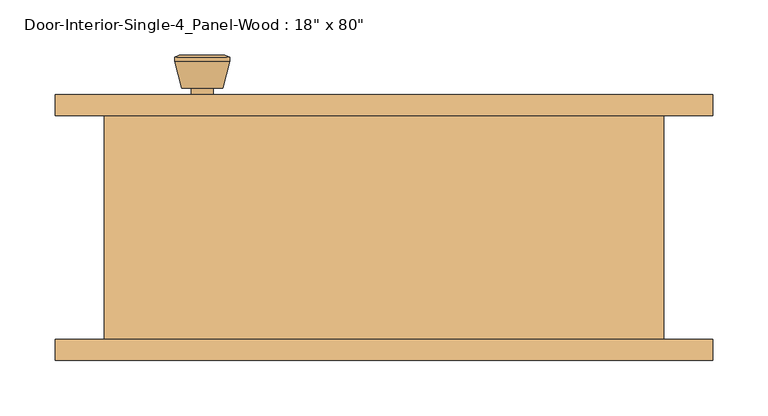
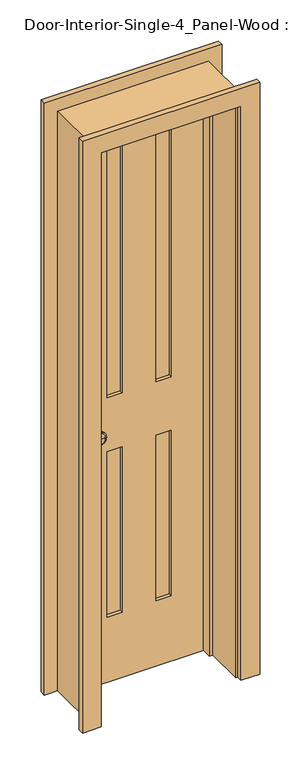
"""IFC4 building model written with IfcOpenShell, lengths in millimetres: door geometry."""

from ifc_helpers import new_model, si_unit, point, frame, frame_2d, origin, place, context, project, spatial, polyline, circle_curve, trimmed, segment, composite_curve, outline, extrude, faceted_brep, source, transform, mapped, element, save
from ifc_brep_helpers import plane_surface, cylinder_surface, revolved_surface, advanced_brep


def door_14995b39(model_context):
    return source(origin(), model_context, "Body", "SolidModel", [
        advanced_brep(
        [(-165.1, 57.5, 914.4), (-155.1, 57.5, 914.4), (-175.1, 57.5, 914.4), (-144.6241324, 8.5, 914.4), (-165.1, 8.5, 914.4), (-185.5758676, 8.5, 914.4), (-140.1, 10.3278681, 914.4), (-190.1, 10.3278681, 914.4), (-140.1, 13.7915463, 914.4), (-190.1, 13.7915463, 914.4), (-146.463764, 38.5, 914.4), (-183.736236, 38.5, 914.4), (-155.1, 38.5, 914.4), (-175.1, 38.5, 914.4)],
        [
            (0, 1),
            (1, 2, circle_curve(frame((-165.1, 57.5, 914.4), z_axis=(0.0, 1.0, 0.0), x_axis=(-1.0, 0.0, 0.0)), 10.0)),
            (2, 0),
            (2, 1, circle_curve(frame((-165.1, 57.5, 914.4), z_axis=(0.0, 1.0, 0.0), x_axis=(-1.0, 0.0, 0.0)), 10.0)),
            (3, 4),
            (4, 5),
            (5, 3, circle_curve(frame((-165.1, 8.5, 914.4), z_axis=(0.0, -1.0, 0.0), x_axis=(-1.0, 0.0, 0.0)), 20.4758676)),
            (3, 5, circle_curve(frame((-165.1, 8.5, 914.4), z_axis=(0.0, -1.0, 0.0), x_axis=(-1.0, 0.0, 0.0)), 20.4758676)),
            (6, 3),
            (5, 7),
            (7, 6, circle_curve(frame((-165.1, 10.3278681, 914.4), z_axis=(0.0, -1.0, 0.0), x_axis=(-1.0, 0.0, 0.0)), 25.0)),
            (6, 7, circle_curve(frame((-165.1, 10.3278681, 914.4), z_axis=(0.0, -1.0, 0.0), x_axis=(-1.0, 0.0, 0.0)), 25.0)),
            (8, 6),
            (7, 9),
            (9, 8, circle_curve(frame((-165.1, 13.7915463, 914.4), z_axis=(0.0, -1.0, 0.0), x_axis=(-1.0, 0.0, 0.0)), 25.0)),
            (8, 9, circle_curve(frame((-165.1, 13.7915463, 914.4), z_axis=(0.0, -1.0, 0.0), x_axis=(-1.0, 0.0, 0.0)), 25.0)),
            (10, 8),
            (9, 11),
            (11, 10, circle_curve(frame((-165.1, 38.5, 914.4), z_axis=(0.0, -1.0, 0.0), x_axis=(-1.0, 0.0, 0.0)), 18.636236)),
            (10, 11, circle_curve(frame((-165.1, 38.5, 914.4), z_axis=(0.0, -1.0, 0.0), x_axis=(-1.0, 0.0, 0.0)), 18.636236)),
            (12, 10),
            (11, 13),
            (13, 12, circle_curve(frame((-165.1, 38.5, 914.4), z_axis=(0.0, -1.0, 0.0), x_axis=(-1.0, 0.0, 0.0)), 10.0)),
            (12, 13, circle_curve(frame((-165.1, 38.5, 914.4), z_axis=(0.0, -1.0, 0.0), x_axis=(-1.0, 0.0, 0.0)), 10.0)),
            (1, 12),
            (13, 2),
        ],
        [
            plane_surface(frame((-165.1, 57.5, 914.4), z_axis=(0.0, 1.0, 0.0), x_axis=(-1.0, 0.0, 0.0))),
            plane_surface(frame((-165.1, 8.5, 914.4), z_axis=(0.0, -1.0, 0.0), x_axis=(-1.0, 0.0, 0.0))),
            revolved_surface(polyline([(-185.5758676, 8.5, 914.4), (-190.1, 10.3278681, 914.4)]), (-165.1, 57.5, 914.4), (0.0, 1.0, 0.0)),
            cylinder_surface(frame((-165.1, 57.5, 914.4), z_axis=(0.0, 1.0, 0.0), x_axis=(-1.0, 0.0, 0.0)), 25.0),
            revolved_surface(polyline([(-190.1, 13.7915463, 914.4), (-183.736236, 38.5, 914.4)]), (-165.1, 57.5, 914.4), (0.0, 1.0, 0.0)),
            plane_surface(frame((-165.1, 38.5, 914.4), z_axis=(0.0, 1.0, 0.0), x_axis=(-1.0, 0.0, 0.0))),
            cylinder_surface(frame((-165.1, 57.5, 914.4), z_axis=(0.0, 1.0, 0.0), x_axis=(-1.0, 0.0, 0.0)), 10.0),
        ],
        [
            (0, [[1, 2, 3]]),
            (0, [[-3, 4, -1]]),
            (1, [[5, 6, 7]]),
            (1, [[-6, -5, 8]]),
            (2, [[9, -7, 10, 11]]),
            (2, [[-10, -8, -9, 12]]),
            (3, [[13, -11, 14, 15]]),
            (3, [[-14, -12, -13, 16]]),
            (4, [[17, -15, 18, 19]]),
            (4, [[-18, -16, -17, 20]]),
            (5, [[21, -19, 22, 23]]),
            (5, [[-22, -20, -21, 24]]),
            (6, [[25, -23, 26, -2]]),
            (6, [[-26, -24, -25, -4]]),
        ],
    ),
        extrude(outline(composite_curve([segment(trimmed(circle_curve(frame_2d((914.4, -165.1)), 30.0), [point((914.4, -195.1))], [point((914.4, -135.1))], False, "CARTESIAN"), True, "CONTINUOUS"), segment(trimmed(circle_curve(frame_2d((914.4, -165.1)), 30.0), [point((914.4, -135.1))], [point((914.4, -195.1))], False, "CARTESIAN"), True, "CONTINUOUS")], self_intersect=False)), frame((0.0, 57.5, 0.0), z_axis=(0.0, 1.0, 0.0), x_axis=(0.0, 0.0, 1.0)), (0.0, 0.0, 1.0), 6.0),
        advanced_brep(
        [(-165.1, 104.425, 914.4), (-175.1, 104.425, 914.4), (-155.1, 104.425, 914.4), (-144.6241324, 153.425, 914.4), (-185.5758676, 153.425, 914.4), (-165.1, 153.425, 914.4), (-140.1, 151.5971319, 914.4), (-190.1, 151.5971319, 914.4), (-140.1, 148.1334537, 914.4), (-190.1, 148.1334537, 914.4), (-146.463764, 123.425, 914.4), (-183.736236, 123.425, 914.4), (-155.1, 123.425, 914.4), (-175.1, 123.425, 914.4)],
        [
            (0, 1),
            (1, 2, circle_curve(frame((-165.1, 104.425, 914.4), z_axis=(0.0, -1.0, 0.0), x_axis=(-1.0, 0.0, 0.0)), 10.0)),
            (2, 0),
            (2, 1, circle_curve(frame((-165.1, 104.425, 914.4), z_axis=(0.0, -1.0, 0.0), x_axis=(-1.0, 0.0, 0.0)), 10.0)),
            (3, 4, circle_curve(frame((-165.1, 153.425, 914.4), z_axis=(0.0, 1.0, 0.0), x_axis=(-1.0, 0.0, 0.0)), 20.4758676)),
            (4, 5),
            (5, 3),
            (4, 3, circle_curve(frame((-165.1, 153.425, 914.4), z_axis=(0.0, 1.0, 0.0), x_axis=(-1.0, 0.0, 0.0)), 20.4758676)),
            (6, 7, circle_curve(frame((-165.1, 151.5971319, 914.4), z_axis=(0.0, 1.0, 0.0), x_axis=(-1.0, 0.0, 0.0)), 25.0)),
            (7, 4),
            (3, 6),
            (7, 6, circle_curve(frame((-165.1, 151.5971319, 914.4), z_axis=(0.0, 1.0, 0.0), x_axis=(-1.0, 0.0, 0.0)), 25.0)),
            (8, 9, circle_curve(frame((-165.1, 148.1334537, 914.4), z_axis=(0.0, 1.0, 0.0), x_axis=(-1.0, 0.0, 0.0)), 25.0)),
            (9, 7),
            (6, 8),
            (9, 8, circle_curve(frame((-165.1, 148.1334537, 914.4), z_axis=(0.0, 1.0, 0.0), x_axis=(-1.0, 0.0, 0.0)), 25.0)),
            (10, 11, circle_curve(frame((-165.1, 123.425, 914.4), z_axis=(0.0, 1.0, 0.0), x_axis=(-1.0, 0.0, 0.0)), 18.636236)),
            (11, 9),
            (8, 10),
            (11, 10, circle_curve(frame((-165.1, 123.425, 914.4), z_axis=(0.0, 1.0, 0.0), x_axis=(-1.0, 0.0, 0.0)), 18.636236)),
            (12, 13, circle_curve(frame((-165.1, 123.425, 914.4), z_axis=(0.0, 1.0, 0.0), x_axis=(-1.0, 0.0, 0.0)), 10.0)),
            (13, 11),
            (10, 12),
            (13, 12, circle_curve(frame((-165.1, 123.425, 914.4), z_axis=(0.0, 1.0, 0.0), x_axis=(-1.0, 0.0, 0.0)), 10.0)),
            (1, 13),
            (12, 2),
        ],
        [
            plane_surface(frame((-165.1, 104.425, 914.4), z_axis=(0.0, -1.0, 0.0), x_axis=(-1.0, 0.0, 0.0))),
            plane_surface(frame((-165.1, 153.425, 914.4), z_axis=(0.0, 1.0, 0.0), x_axis=(-1.0, 0.0, 0.0))),
            revolved_surface(polyline([(-185.5758676, 153.425, 914.4), (-190.1, 151.5971319, 914.4)]), (-165.1, 104.425, 914.4), (0.0, -1.0, 0.0)),
            cylinder_surface(frame((-165.1, 104.425, 914.4), z_axis=(0.0, -1.0, 0.0), x_axis=(-1.0, 0.0, 0.0)), 25.0),
            revolved_surface(polyline([(-190.1, 148.1334537, 914.4), (-183.736236, 123.425, 914.4)]), (-165.1, 104.425, 914.4), (0.0, -1.0, 0.0)),
            plane_surface(frame((-165.1, 123.425, 914.4), z_axis=(0.0, -1.0, 0.0), x_axis=(-1.0, 0.0, 0.0))),
            cylinder_surface(frame((-165.1, 104.425, 914.4), z_axis=(0.0, -1.0, 0.0), x_axis=(-1.0, 0.0, 0.0)), 10.0),
        ],
        [
            (0, [[1, 2, 3]]),
            (0, [[-3, 4, -1]]),
            (1, [[5, 6, 7]]),
            (1, [[8, -7, -6]]),
            (2, [[9, 10, -5, 11]]),
            (2, [[12, -11, -8, -10]]),
            (3, [[13, 14, -9, 15]]),
            (3, [[16, -15, -12, -14]]),
            (4, [[17, 18, -13, 19]]),
            (4, [[20, -19, -16, -18]]),
            (5, [[21, 22, -17, 23]]),
            (5, [[24, -23, -20, -22]]),
            (6, [[-2, 25, -21, 26]]),
            (6, [[-4, -26, -24, -25]]),
        ],
    ),
        extrude(outline(composite_curve([segment(trimmed(circle_curve(frame_2d((914.4, -165.1)), 30.0), [point((914.4, -195.1))], [point((914.4, -135.1))], False, "CARTESIAN"), True, "CONTINUOUS"), segment(trimmed(circle_curve(frame_2d((914.4, -165.1)), 30.0), [point((914.4, -135.1))], [point((914.4, -195.1))], False, "CARTESIAN"), True, "CONTINUOUS")], self_intersect=False)), frame((0.0, 98.425, 0.0), z_axis=(0.0, 1.0, 0.0), x_axis=(0.0, 0.0, 1.0)), (0.0, 0.0, 1.0), 6.0),
        extrude(outline(polyline([(107.95, 75.1416667), (57.15, 75.1416667), (57.15, 86.7833333), (107.95, 86.7833333), (107.95, 75.1416667)])), frame((0.0, 0.0, 1009.65), z_axis=(0.0, 0.0, 1.0), x_axis=(1.0, 0.0, 0.0)), (0.0, 0.0, 1.0), 903.2875),
        extrude(outline(polyline([(-57.15, 75.1416667), (-107.95, 75.1416667), (-107.95, 86.7833333), (-57.15, 86.7833333), (-57.15, 75.1416667)])), frame((0.0, 0.0, 1009.65), z_axis=(0.0, 0.0, 1.0), x_axis=(1.0, 0.0, 0.0)), (0.0, 0.0, 1.0), 903.2875),
        extrude(outline(polyline([(107.95, 75.1416667), (57.15, 75.1416667), (57.15, 86.7833333), (107.95, 86.7833333), (107.95, 75.1416667)])), frame((0.0, 0.0, 231.775), z_axis=(0.0, 0.0, 1.0), x_axis=(1.0, 0.0, 0.0)), (0.0, 0.0, 1.0), 587.375),
        extrude(outline(polyline([(-57.15, 75.1416667), (-107.95, 75.1416667), (-107.95, 86.7833333), (-57.15, 86.7833333), (-57.15, 75.1416667)])), frame((0.0, 0.0, 231.775), z_axis=(0.0, 0.0, 1.0), x_axis=(1.0, 0.0, 0.0)), (0.0, 0.0, 1.0), 587.375),
        extrude(outline(polyline([(2032.0, -228.6), (0.0, -228.6), (0.0, 228.6), (2032.0, 228.6), (2032.0, -228.6)]), holes=[polyline([(1912.9375, 57.15), (1912.9375, 107.95), (1009.65, 107.95), (1009.65, 57.15), (1912.9375, 57.15)]), polyline([(1009.65, -57.15), (1009.65, -107.95), (1912.9375, -107.95), (1912.9375, -57.15), (1009.65, -57.15)]), polyline([(819.15, 57.15), (819.15, 107.95), (231.775, 107.95), (231.775, 57.15), (819.15, 57.15)]), polyline([(231.775, -57.15), (231.775, -107.95), (819.15, -107.95), (819.15, -57.15), (231.775, -57.15)])]), frame((0.0, 63.5, 0.0), z_axis=(0.0, 1.0, 0.0), x_axis=(0.0, 0.0, 1.0)), (0.0, 0.0, 1.0), 34.925),
        faceted_brep([(254.0, 98.425, 0.0), (254.0, -104.775, 0.0), (228.6, -104.775, 0.0), (228.6, 28.575, 0.0), (215.9, 28.575, 0.0), (215.9, 63.5, 0.0), (228.6, 63.5, 0.0), (228.6, 98.425, 0.0), (254.0, 98.425, 2057.4), (254.0, -104.775, 2057.4), (-254.0, -104.775, 2057.4), (-254.0, -104.775, 0.0), (-228.6, -104.775, 0.0), (-228.6, -104.775, 2032.0), (228.6, -104.775, 2032.0), (228.6, 28.575, 2032.0), (-228.6, 28.575, 2032.0), (-228.6, 28.575, 0.0), (-215.9, 28.575, 0.0), (-215.9, 28.575, 2019.3), (215.9, 28.575, 2019.3), (215.9, 63.5, 2019.3), (-215.9, 63.5, 2019.3), (-215.9, 63.5, 0.0), (-228.6, 63.5, 0.0), (-228.6, 63.5, 2032.0), (228.6, 63.5, 2032.0), (228.6, 98.425, 2032.0), (-228.6, 98.425, 2032.0), (-228.6, 98.425, 0.0), (-254.0, 98.425, 0.0), (-254.0, 98.425, 2057.4)], [[[0, 1, 2, 3, 4, 5, 6, 7]], [[1, 0, 8, 9]], [[2, 1, 9, 10, 11, 12, 13, 14]], [[3, 2, 14, 15]], [[4, 3, 15, 16, 17, 18, 19, 20]], [[5, 4, 20, 21]], [[6, 5, 21, 22, 23, 24, 25, 26]], [[7, 6, 26, 27]], [[0, 7, 27, 28, 29, 30, 31, 8]], [[9, 8, 31, 10]], [[15, 14, 13, 16]], [[21, 20, 19, 22]], [[27, 26, 25, 28]], [[30, 29, 24, 23, 18, 17, 12, 11]], [[10, 31, 30, 11]], [[16, 13, 12, 17]], [[22, 19, 18, 23]], [[28, 25, 24, 29]]]),
        extrude(outline(polyline([(0.0, 234.95), (0.0, 298.45), (2101.85, 298.45), (2101.85, -298.45), (0.0, -298.45), (0.0, -234.95), (2038.35, -234.95), (2038.35, 234.95), (0.0, 234.95)])), frame((0.0, -123.825, 0.0), z_axis=(0.0, 1.0, 0.0), x_axis=(0.0, 0.0, 1.0)), (0.0, 0.0, 1.0), 19.05),
        extrude(outline(polyline([(0.0, 234.95), (0.0, 298.45), (2101.85, 298.45), (2101.85, -298.45), (0.0, -298.45), (0.0, -234.95), (2038.35, -234.95), (2038.35, 234.95), (0.0, 234.95)])), frame((0.0, 98.425, 0.0), z_axis=(0.0, 1.0, 0.0), x_axis=(0.0, 0.0, 1.0)), (0.0, 0.0, 1.0), 19.05),
    ])


if __name__ == "__main__":
    model = new_model("IFC4")
    model_context = context("Model", 3, world=origin())
    ifc_project = project(units=[si_unit("LENGTHUNIT", "METRE", prefix="MILLI")], contexts=[model_context])
    site = spatial("IfcSite", under=ifc_project)
    building = spatial("IfcBuilding", under=site)
    placement = place(None, origin())
    door_shape = door_14995b39(model_context)
    element("IfcDoor", 1, ObjectType="Door-Interior-Single-4_Panel-Wood : 18\" x 80\"", at=placement, inside=building, context=model_context, shape_type="MappedRepresentation", body=[
        mapped(door_shape, transform((0.0, 0.0, 0.0), x_axis=(1.0, 0.0, 0.0), y_axis=(0.0, 1.0, 0.0), z_axis=(0.0, 0.0, 1.0))),
    ])
    save(model, "model.ifc")

# Revit data of these elements
# Type "Door-Interior-Single-4_Panel-Wood : 18\" x 80\""
#   Type Mark = "8"
#   Assembly Code = "C1020300"
#   Analytic Construction = "Wooden"
#   Top Rail = 0' - 4 11/16"
#   Thickness = 0' - 1 3/8"
#   Thermal Resistance (R) = 2.5876 (h·ft²·°F)/BTU
#   Swing Angle [instance default] = 90.00°
#   Stiles = 0' - 4 3/4"
#   Rough Width = 1' - 8"
#   Rough Height = 6' - 9"
#   Mullion = 0' - 4 1/2"
#   Lock Rail = 0' - 7 1/2"
#   Height = 6' - 8"
#   Width = 1' - 6"
#   Heat Transfer Coefficient (U) = 0.3865 BTU/(h·ft²·°F)
#   Bottom Rail = 0' - 9 1/8"
#   Trim Material = Cherry
#   Panel Material = Cherry
#   Frame Material = Cherry
#   Door Handle Material = Aluminum
#   Visual Light Transmittance = 0
#   Solar Heat Gain Coefficient = 0
#   Wall Closure = (empty or 0)
#   Function = (empty or 0)
# Element 1 (IfcDoor, "Door-Interior-Single-4_Panel-Wood : 18\" x 80\"")
#   Materials on its faces: "Cherry", "Aluminum"
# Materials
#   "Cherry": class "Wood", colour RGB 226 177 128, transparency 0, Description = "Prunus Serotina", Cost = 0
#   "Aluminum": class "Metal", colour RGB 247 247 247, transparency 0, Description = "Aluminum 6061", Cost = 0
